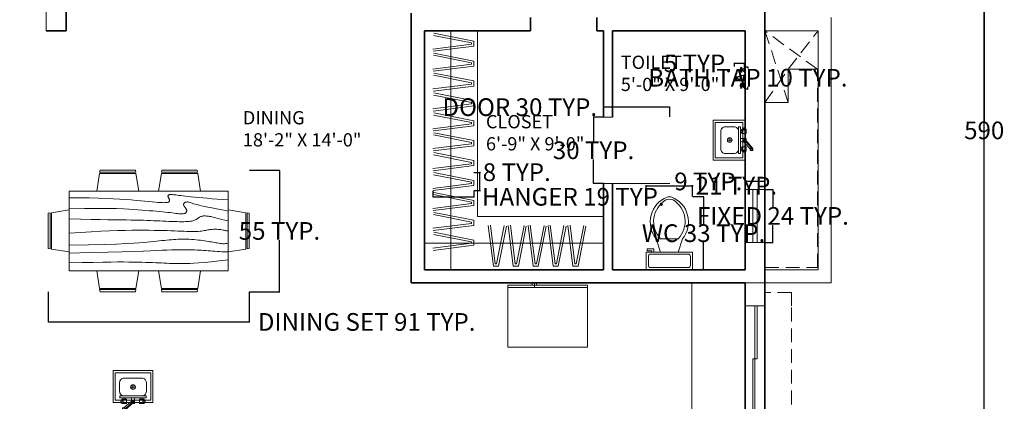
# Model space of a CAD drawing. Units: inches. Extents: x 3343 to 4790, y 1140 to 2641.
# Tile 9 of 10: x 4337 to 4782, y 2024 to 2196. Entities that reach past the tile are written whole.
import ezdxf

# ---------------------------------------------------------------- set-up
doc = ezdxf.new("R2010")
doc.units = ezdxf.units.IN
doc.header["$LTSCALE"] = 5
doc.header["$MEASUREMENT"] = 0
doc.linetypes.add('HIDDEN', pattern=[0.375, 0.25, -0.125])
for name, color, linetype, lineweight in [('A-ANNO-DIMS', 2, 'Continuous', 18), ('A-AREA-IDEN', 7, 'Continuous', 18), ('A-DOOR', 3, 'Continuous', 18), ('A-EQPM', 9, 'Continuous', 18), ('A-FLOR-CASE', 9, 'Continuous', 18), ('A-FLOR-FIXT', 9, 'Continuous', 18), ('A-FLOR-HIDN', 8, 'HIDDEN', 13), ('A-FLOR-SHFT', 8, 'Continuous', 18), ('A-FURN', 8, 'Continuous', 13), ('A-GLAZ', 4, 'Continuous', 18), ('A-WALL', 7, 'Continuous', 35)]:
    doc.layers.add(name, color=color, linetype=linetype, lineweight=lineweight)
doc.styles.get("Standard").update_dxf_attribs({"font": 'arial.ttf'})
doc.dimstyles.get("Standard").update_dxf_attribs({"dimtxt": 8, "dimasz": 0.18, "dimexe": 0.18, "dimexo": 0.0625, "dimgap": 0.09, "dimtad": 0, "dimtih": 1, "dimtoh": 1, "dimdec": 1, "dimzin": 0, "dimdsep": 46, "dimlunit": 3, "dimtxsty": 'Standard', "dimcen": 0.09, "dimadec": 0, "dimazin": 0, "dimtfac": 1, "dimtdec": 1, "dimtofl": 0, "dimtmove": 0, "dimatfit": 3, "dimfxl": 1, "dimtolj": 1, "dimtzin": 0, "dimarcsym": 0})

# ---------------------------------------------------------------- blocks, each defined once
blk = doc.blocks.new('Dining Set - 36 x 72 in.')
for p, q in [((-22, 27.5), (-22.1562, 26.50042)), ((-22, 27.5), (-6, 27.5)), ((-5.8437, 26.49966), (-6, 27.5)), ((6, 27.5), (5.8438, 26.50042)), ((6, 27.5), (22, 27.5)), ((22.1563, 26.49966), (22, 27.5)), ((-22.2343, 26.00059), (-23.4847, 17.99762)), ((-22.2304, 26), (-5.7608, 26)), ((-5.8416, 26.5), (-22.1534, 26.5)), ((-4.5152, 17.99762), (-5.7655, 25.99926)), ((5.7657, 26.00059), (4.5153, 17.99762)), ((5.7696, 26), (22.2392, 26)), ((22.1584, 26.5), (5.8466, 26.5)), ((23.4848, 17.99762), (22.2345, 25.99926)), ((36, 18), (-36, 18)), ((-36, 18), (-36, -18)), ((36, -18), (36, 18)), ((-44.0006, 8.23428), (-35.9976, 9.48474)), ((44.0006, 8.23428), (35.9976, 9.48474)), ((-45.5, 8), (-44.5004, 8.15617)), ((-45.5, 8), (-45.5, -8)), ((-44.5, -8.15843), (-44.5, 8.15338)), ((-44, 8.23041), (-44, -8.23915)), ((44, 8.23041), (44, -8.23915)), ((44.5, -8.15843), (44.5, 8.15338)), ((45.5, 8), (44.5005, 8.15617)), ((45.5, 8), (45.5, -8)), ((-44.4997, -8.15631), (-45.5, -8)), ((-35.9976, -9.48476), (-43.9993, -8.2345)), ((35.9976, -9.48476), (43.9993, -8.2345)), ((44.4997, -8.15631), (45.5, -8)), ((-36, -18), (36, -18)), ((-22.2343, -26.0006), (-23.4847, -17.99762)), ((-4.5152, -17.99762), (-5.7655, -25.99928)), ((5.7657, -26.0006), (4.5153, -17.99762)), ((23.4848, -17.99762), (22.2345, -25.99928)), ((-22.2304, -26), (-5.7608, -26)), ((-22, -27.5), (-22.1562, -26.50044)), ((-5.8416, -26.5), (-22.1534, -26.5)), ((-5.8437, -26.49967), (-6, -27.5)), ((5.7696, -26), (22.2392, -26)), ((6, -27.5), (5.8438, -26.50044)), ((22.1584, -26.5), (5.8466, -26.5)), ((22.1563, -26.49967), (22, -27.5)), ((-22, -27.5), (-6, -27.5)), ((6, -27.5), (22, -27.5))]:
    blk.add_line(p, q)
for points in [[(-36, 15), (-31.1772, 14.97754), (-26.8079, 14.91406), (-22.8538, 14.81543), (-19.276, 14.6875), (-16.0362, 14.53613), (-13.0957, 14.36718), (-10.4159, 14.18652), (-7.9583, 14), (-5.6904, 13.81315), (-3.6035, 13.63021), (-1.6954, 13.45508), (0.0365, 13.29166), (1.5945, 13.14388), (2.9811, 13.01562), (4.1988, 12.9108), (5.25, 12.83333), (6.1393, 12.78613), (6.8802, 12.76823), (7.4883, 12.77767), (7.9792, 12.8125), (8.3685, 12.87077), (8.6719, 12.95052), (8.9049, 13.0498), (9.0833, 13.16666), (9.2205, 13.29899), (9.3216, 13.44401), (9.3895, 13.59879), (9.4271, 13.76041), (9.4373, 13.92594), (9.4232, 14.09245), (9.3875, 14.257), (9.3333, 14.41666), (9.2638, 14.56917), (9.1836, 14.71484), (9.0975, 14.85465), (9.0104, 14.98958), (8.9272, 15.1206), (8.8529, 15.2487), (8.7922, 15.37483), (8.75, 15.5), (8.7305, 15.62467), (8.7344, 15.74739), (8.7617, 15.86621), (8.8125, 15.97916), (8.8867, 16.08431), (8.9844, 16.17968), (9.1055, 16.26334), (9.25, 16.33333), (9.4189, 16.38802), (9.6172, 16.42708), (9.8506, 16.45052), (10.125, 16.45833), (10.4463, 16.45052), (10.8203, 16.42708), (11.2529, 16.38802), (11.75, 16.33333), (12.3184, 16.26318), (12.9694, 16.17838), (13.7151, 16.07991), (14.5677, 15.96875), (15.5395, 15.84586), (16.6426, 15.71224), (17.8893, 15.56884), (19.2917, 15.41666), (20.859, 15.25667), (22.5879, 15.08984), (24.4721, 14.91715), (26.5052, 14.73958), (28.6809, 14.5581), (30.9929, 14.3737), (33.4347, 14.18733), (36, 14)], [(-36, 10), (-28.9766, 10.14274), (-23.1725, 10.20442), (-18.4241, 10.19775), (-14.5677, 10.13541), (-11.4399, 10.03011), (-8.877, 9.89453), (-6.7154, 9.74137), (-4.7917, 9.58333), (-2.9698, 9.43082), (-1.2246, 9.28515), (0.4415, 9.14534), (2.026, 9.01041), (3.5266, 8.87939), (4.9408, 8.7513), (6.266, 8.62516), (7.5, 8.5), (8.6411, 8.37549), (9.6914, 8.2539), (10.6538, 8.13818), (11.5312, 8.03125), (12.3267, 7.93603), (13.043, 7.85547), (13.6831, 7.79248), (14.25, 7.75), (14.7471, 7.7303), (15.1797, 7.73307), (15.5537, 7.75732), (15.875, 7.80208), (16.1494, 7.86637), (16.3828, 7.94922), (16.5811, 8.04964), (16.75, 8.16666), (16.8944, 8.29915), (17.0143, 8.44531), (17.1089, 8.60319), (17.1771, 8.77083), (17.218, 8.94629), (17.2305, 9.1276), (17.2137, 9.31282), (17.1667, 9.5), (17.0895, 9.6875), (16.987, 9.875), (16.8649, 10.0625), (16.7292, 10.25), (16.5856, 10.4375), (16.4401, 10.625), (16.2985, 10.8125), (16.1667, 11), (16.05, 11.18733), (15.9518, 11.3737), (15.8752, 11.5581), (15.8229, 11.73958), (15.798, 11.91715), (15.8034, 12.08984), (15.842, 12.25667), (15.9167, 12.41666), (16.0295, 12.56836), (16.1784, 12.70833), (16.3605, 12.83268), (16.5729, 12.9375), (16.8127, 13.01888), (17.0768, 13.07291), (17.3625, 13.0957), (17.6667, 13.08333), (17.9894, 13.03312), (18.3418, 12.94726), (18.7382, 12.82918), (19.1927, 12.68229), (19.7195, 12.51001), (20.3327, 12.31575), (21.0465, 12.10294), (21.875, 11.875), (22.8357, 11.63354), (23.959, 11.37304), (25.2786, 11.08618), (26.8282, 10.76562), (28.6414, 10.40405), (30.752, 9.99414), (33.1936, 9.52856), (36, 9)], [(-36, 5.5), (-30.7157, 5.3348), (-26.069, 5.20963), (-21.9946, 5.11767), (-18.4271, 5.05208), (-15.3009, 5.00602), (-12.5508, 4.97265), (-10.1112, 4.94515), (-7.9167, 4.91666), (-5.909, 4.88167), (-4.0586, 4.83984), (-2.3429, 4.79215), (-0.7396, 4.73958), (0.7739, 4.6831), (2.22, 4.6237), (3.6213, 4.56233), (5, 4.5), (6.373, 4.43782), (7.7344, 4.3776), (9.0723, 4.32129), (10.375, 4.27083), (11.6309, 4.22819), (12.8281, 4.19531), (13.9551, 4.17415), (15, 4.16666), (15.954, 4.17448), (16.819, 4.19791), (17.6001, 4.23698), (18.3021, 4.29166), (18.9299, 4.36198), (19.4883, 4.44791), (19.9823, 4.54948), (20.4167, 4.66666), (20.7969, 4.79899), (21.1302, 4.94401), (21.4245, 5.09879), (21.6875, 5.26041), (21.9271, 5.42594), (22.1511, 5.59245), (22.3672, 5.757), (22.5834, 5.91666), (22.8065, 6.06868), (23.0404, 6.21093), (23.2879, 6.34147), (23.5521, 6.45833), (23.8358, 6.55957), (24.142, 6.64323), (24.4735, 6.70735), (24.8334, 6.75), (25.2235, 6.76969), (25.642, 6.76692), (26.0858, 6.74267), (26.5521, 6.69791), (27.0379, 6.63362), (27.5404, 6.55078), (28.0565, 6.45036), (28.5834, 6.33333), (29.1242, 6.19987), (29.7071, 6.04687), (30.3661, 5.87044), (31.1354, 5.66666), (32.0493, 5.43164), (33.142, 5.16146), (34.4475, 4.85221), (36, 4.5)], [(-36, -1), (-30.7915, -0.6591), (-26.0195, -0.38216), (-21.6519, -0.16284), (-17.6563, 0.00521), (-14.0005, 0.12833), (-10.6523, 0.21289), (-7.5796, 0.26522), (-4.75, 0.29166), (-2.134, 0.29793), (0.2878, 0.28711), (2.5317, 0.26163), (4.6146, 0.22396), (6.5529, 0.17651), (8.3633, 0.12174), (10.0623, 0.06209), (11.6667, 0), (13.1899, -0.06201), (14.6341, -0.1211), (15.9982, -0.17432), (17.2813, -0.21875), (18.4823, -0.25147), (19.6003, -0.26953), (20.6343, -0.27002), (21.5834, -0.25), (22.4481, -0.20768), (23.2357, -0.14584), (23.9549, -0.06836), (24.6146, 0.02083), (25.2235, 0.11784), (25.7904, 0.21875), (26.3241, 0.31966), (26.8334, 0.41666), (27.3265, 0.50618), (27.8099, 0.58593), (28.2894, 0.65397), (28.7709, 0.70833), (29.2601, 0.74707), (29.763, 0.76823), (30.2855, 0.76985), (30.8334, 0.75), (31.4088, 0.70784), (31.9994, 0.64713), (32.589, 0.57275), (33.1615, 0.48958), (33.7008, 0.4025), (34.1908, 0.3164), (34.6153, 0.23616), (34.9584, 0.16666), (35.2099, 0.11165), (35.3848, 0.07031), (35.504, 0.04069), (35.5886, 0.02083), (35.6594, 0.00879), (35.7377, 0.0026), (35.8442, 0.00032), (36, 0)], [(-36, -6.5), (-27.1843, -6.31267), (-20.084, -6.1263), (-14.469, -5.9419), (-10.1094, -5.76042), (-6.7752, -5.58285), (-4.2363, -5.41016), (-2.2629, -5.24333), (-0.625, -5.08334), (0.8708, -4.93099), (2.2715, -4.78646), (3.5872, -4.64974), (4.8281, -4.52084), (6.0046, -4.39974), (7.127, -4.28646), (8.2053, -4.18099), (9.25, -4.08334), (10.2705, -3.99382), (11.2734, -3.91407), (12.2647, -3.84603), (13.25, -3.79167), (14.2354, -3.75293), (15.2266, -3.73177), (16.2295, -3.73015), (17.25, -3.75), (18.2912, -3.79248), (19.3451, -3.85547), (20.4009, -3.93604), (21.4479, -4.03125), (22.4754, -4.13819), (23.4727, -4.25391), (24.4289, -4.37549), (25.3334, -4.5), (26.1785, -4.62492), (26.9694, -4.74935), (27.7145, -4.87281), (28.4219, -4.99479), (29.1, -5.11483), (29.7572, -5.23242), (30.4016, -5.34709), (31.0417, -5.45834), (31.6837, -5.56437), (32.3262, -5.65821), (32.9658, -5.73153), (33.599, -5.77604), (34.2224, -5.78345), (34.8327, -5.74545), (35.4264, -5.65373), (36, -5.5)], [(-36, -10), (-26.4022, -9.81299), (-18.4675, -9.62891), (-11.9839, -9.45069), (-6.7396, -9.28125), (-2.5226, -9.12354), (0.8789, -8.98047), (3.6769, -8.85498), (6.0833, -8.75), (8.2767, -8.66765), (10.3021, -8.60677), (12.1712, -8.56543), (13.8958, -8.54167), (15.4876, -8.53353), (16.9583, -8.53907), (18.3197, -8.55632), (19.5834, -8.58334), (20.7616, -8.61841), (21.8685, -8.66081), (22.9188, -8.71004), (23.9271, -8.76563), (24.9081, -8.82707), (25.8763, -8.89388), (26.8465, -8.96558), (27.8334, -9.04167), (28.8474, -9.12118), (29.8828, -9.20117), (30.93, -9.27824), (31.9792, -9.34896), (33.0205, -9.40991), (34.0443, -9.45768), (35.0407, -9.48885), (36, -9.5)], [(-36, -14.5), (-30.0881, -14.33513), (-25.0332, -14.21224), (-20.7312, -14.12647), (-17.0781, -14.07292), (-13.97, -14.04671), (-11.3027, -14.04297), (-8.9724, -14.05681), (-6.875, -14.08334), (-4.9224, -14.11833), (-3.0905, -14.16016), (-1.3709, -14.20785), (0.2448, -14.26042), (1.7647, -14.3169), (3.1973, -14.3763), (4.5507, -14.43767), (5.8333, -14.5), (7.0554, -14.5621), (8.235, -14.62175), (9.3922, -14.67652), (10.5469, -14.72396), (11.7192, -14.76164), (12.929, -14.78711), (14.1965, -14.79794), (15.5417, -14.79167), (16.9933, -14.76424), (18.6152, -14.70508), (20.4804, -14.60197), (22.6615, -14.44271), (25.2312, -14.21509), (28.2624, -13.9069), (31.8277, -13.50594), (36, -13)]]:
    blk.add_lwpolyline(points)
blk = doc.blocks.new('Toilet - top')
for p, q in [((9.5, -6), (9.5, -2)), ((-10, -8.5), (-8, -8.5)), ((-10, -9.5), (-10, -8.5)), ((-8, -8.5), (-8, -8)), ((-7, -8), (-7, -9.5)), ((-4, -8), (-6, -14)), ((4, -8), (6, -14)), ((-7, -9.5), (-10, -9.5)), ((4, -14), (-4, -14))]:
    blk.add_line(p, q)
blk.add_lwpolyline([(10.5, -8), (10.5, 0), (-10.5, 0), (-10.5, -8)], close=True)
for points in [[(-9.5, -2), (-9.5, -6)], [(8.5, -1), (-8.5, -1)], [(-8.5, -7), (8.5, -7)]]:
    blk.add_lwpolyline(points)
for centre, radius, start, end in [((-8.62, -1.88), 0.884, 81.8699, 188.1301), ((8.62, -1.88), 0.884, 351.8699, 98.1301), ((-8.62, -6.12), 0.884, 171.8699, 278.1301), ((8.62, -6.12), 0.884, 261.8699, 8.1301), ((3.52, -21.58), 12.17, 141.4691, 247.9714), ((4.2, -21.82), 11.33, 136.3677, 238.9468), ((-3.52, -21.58), 12.17, 292.0284, 38.5307), ((-4.2, -21.82), 11.33, 301.053, 43.6321), ((0, -27.88), 4, 245.7318, 294.2682), ((0, -29), 4, 254.8605, 285.1395)]:
    blk.add_arc(centre, radius, start, end)
blk = doc.blocks.new('Faucet - Bathroom front')
for p, q in [((-5, 0), (-2.25, 0)), ((-4.5087, 0.25), (-2.7408, 0.25)), ((-4, 1.625), (-4.25, 1.625)), ((-4, 1.375), (-4.25, 1.375)), ((-3.1442, 0.75), (-4.0979, 0.75)), ((-3.25, 1.625), (-3, 1.625)), ((-3.25, 1.375), (-3, 1.375)), ((-1.5, 0), (1.5, 0)), ((-1, 0.5), (1, 0.5)), ((-0.5, 4.25), (0.5, 4.25)), ((0.5, 3.75), (-0.5, 3.75)), ((-0.5, 3), (0.5, 3)), ((0.5, 2), (-0.5, 2)), ((-0.25, 3), (-0.25, 3.5)), ((0.25, 3.5), (0.25, 3)), ((2.25, 0), (5, 0)), ((2.7413, 0.25), (4.5092, 0.25)), ((3.25, 1.625), (3, 1.625)), ((3.25, 1.375), (3, 1.375)), ((4.1058, 0.75), (3.1521, 0.75)), ((4, 1.625), (4.25, 1.625)), ((4, 1.375), (4.25, 1.375))]:
    blk.add_line(p, q)
for points in [[(-0.25, 4.5), (0.25, 4.5)], [(-0.5, 3.75), (-0.5, 4.25)], [(0.25, 3.5), (-0.25, 3.5)], [(0.5, 4.25), (0.5, 3.75)]]:
    blk.add_lwpolyline(points)
for points in [[(-4, 1), (-4, 2), (-3.25, 2), (-3.25, 1)], [(3.25, 1), (3.25, 2), (4, 2), (4, 1)]]:
    blk.add_lwpolyline(points, close=True)
for centre in [(-4.5, 1.5), (-3.625, 1.5), (-2.75, 1.5), (2.75, 1.5), (3.625, 1.5), (4.5, 1.5)]:
    blk.add_circle(centre, 0.2795)
for centre, radius, start, end in [((-0.2575, 4.2575), 0.2426, 88.22243, 181.7776), ((0.2575, 4.2575), 0.2426, 358.2224, 91.77757), ((-5.375, 1.375), 1.4252, 285.2551, 344.7449), ((-1.875, 1.375), 1.4252, 195.2551, 254.7449), ((-0.7962, -0.2038), 0.7327, 106.1502, 163.8498), ((3, 1), 4.0311, 150.2551, 187.125), ((0.6413, 2.5), 1.246, 156.3417, 203.6583), ((-0.2575, 3.7425), 0.2426, 178.2224, 271.7776), ((0.2575, 3.7425), 0.2426, 268.2224, 1.777565), ((-3, 1), 4.0311, 352.875, 29.74488), ((-0.6413, 2.5), 1.246, 336.3417, 23.65835), ((0.7962, -0.2038), 0.7327, 16.1502, 73.84979), ((1.875, 1.375), 1.4252, 285.2551, 344.7449), ((5.375, 1.375), 1.4252, 195.2551, 254.7449)]:
    blk.add_arc(centre, radius, start, end)
blk = doc.blocks.new('Faucet - kit sink front')
for p, q in [((-0.25, 3), (3.75, 6.5)), ((3.75, 6), (-0.25, 2.5)), ((4.1921, 5.5041), (0.75, 2.5)), ((3.75, 6), (3.75, 6.5)), ((3.75, 6.5), (4.75, 6.5)), ((3.75, 5.5), (3.75, 6)), ((4.75, 6), (3.75, 6)), ((4.75, 5.5), (3.75, 5.5)), ((4.75, 6.5), (4.75, 6)), ((4.75, 6), (4.75, 5.5)), ((-4.5, 1), (-4.5, 1.5)), ((-3.5, 1.5), (-3.5, 1)), ((-0.75, 3.5), (0.3192, 3.5)), ((-0.75, 1), (-0.75, 3.5)), ((-0.25, 2.5), (-0.25, 3)), ((0.75, 2.5), (-0.25, 2.5)), ((0.75, 2.5), (0.75, 1)), ((3.5, 1.5), (3.5, 1)), ((4.5, 1), (4.5, 1.5))]:
    blk.add_line(p, q)
for points in [[(-6, 0), (-6, 1), (6, 1), (6, 0)], [(-5.5, 2.5), (-5.5, 3.25), (-4.5, 3.25), (-4.5, 2.5)], [(5.5, 2.5), (5.5, 3.25), (4.5, 3.25), (4.5, 2.5)]]:
    blk.add_lwpolyline(points, close=True)
for points in [[(-5, 3.2513), (-5, 3.5), (-3, 3.5), (-3, 1.5), (-5, 1.5), (-5, 2.5)], [(5, 3.2513), (5, 3.5), (3, 3.5), (3, 1.5), (5, 1.5), (5, 2.5)]]:
    blk.add_lwpolyline(points)
blk = doc.blocks.new('Refrigerator-2 door - 36 in top')
for p, q in [((0, -26.999999), (36, -26.999999)), ((11, -27.999999), (11, -28.999999)), ((11, -28.999999), (13, -28.999999)), ((12, -26.999999), (12, -28.999999)), ((13, -28.999999), (13, -27.999999))]:
    blk.add_line(p, q)
blk.add_lwpolyline([(0, -27.999999), (0, 0), (36, 0), (36, -27.999999)], close=True)
blk = doc.blocks.new('SINK-BOWL-WITH-DRAIN')
for p, q in [((8.58, 9.03), (6.47, 9.03)), ((7.52, 10.09), (7.52, 7.97))]:
    blk.add_line(p, q)
for points in [[(14.44, 0), (0, 0), (0, 18.06), (14.44, 18.06)], [(1, 1), (1, 17.06), (13.44, 17.06), (13.44, 1)]]:
    blk.add_lwpolyline(points, close=True)
blk.add_lwpolyline([(9.44, 15.06), (5.44, 15.06, 0.414214), (3.44, 13.06), (3.44, 5, 0.414214), (5.44, 3), (9.44, 3, 0.414214), (11.44, 5), (11.44, 13.06, 0.414214)], format="xyb", close=True)
blk.add_circle((7.52, 9.03), 1.06)
blk = doc.blocks.new('WINDOW-48IN-SLIDING-JAMB9')
for p, q in [((0, 9), (0, 0)), ((48, 9), (48, 0)), ((0, 5.5), (24, 5.5)), ((0, 4.5), (48, 4.5)), ((24, 5.5), (24, 3.5)), ((24, 3.5), (48, 3.5))]:
    blk.add_line(p, q)
blk = doc.blocks.new('WINDOW-24IN-FIXED')
for p, q in [((0, 9), (0, 0)), ((24, 9), (24, 0)), ((0, 5.5), (24, 5.5)), ((0, 3.5), (24, 3.5))]:
    blk.add_line(p, q)
blk = doc.blocks.new('DOOR-36IN-6IN-JAMB')
for p, q in [((0, 30), (0, 36)), ((36, 30), (36, 36)), ((36, 36), (36, 0))]:
    blk.add_line(p, q)
blk = doc.blocks.new('DOOR-30IN-4IN-JAMB')
for p, q in [((30, 30), (0, 30)), ((26, 30), (30, 30)), ((26, 0), (30, 0))]:
    blk.add_line(p, q)
blk = doc.blocks.new('WARDROBE-HANGER')
for points in [[(0.22, 7.19), (17.51, 3.78), (17.51, 3.18), (0, 0.99)], [(0.41, 8.17), (18.51, 4.61), (18.51, 2.3), (0.12, 0)]]:
    blk.add_lwpolyline(points)
blk = doc.blocks.new('*D29')
at = {"layer": 'A-ANNO-DIMS', "color": 0, "lineweight": -2, "ltscale": 5, "transparency": 16777216}
for p, q in [((4523.96, 2118.86), (4523.96, 2115.96)), ((4524.14, 2116.14), (4542.3, 2116.14)), ((4542.48, 2118.86), (4542.48, 2115.96)), ((4542.48, 2116.14), (4542.66, 2116.14))]:
    blk.add_line(p, q, dxfattribs=at)
at = {"layer": 'A-ANNO-DIMS', "color": 0, "ltscale": 5, "transparency": 16777216}
for points in [[(4524.14, 2116.17), (4524.14, 2116.11), (4523.96, 2116.14)], [(4542.3, 2116.17), (4542.3, 2116.11), (4542.48, 2116.14)]]:
    blk.add_solid(points, dxfattribs=at)
at = {"layer": 'Defpoints', "color": 0, "ltscale": 5, "transparency": 16777216}
for p in [(4523.96, 2118.92), (4542.48, 2118.92), (4542.48, 2116.14)]:
    blk.add_point(p, dxfattribs=at)
at = {"layer": 'A-ANNO-DIMS', "color": 0, "ltscale": 5, "transparency": 16777216, "insert": (4587.46, 2116.14), "char_height": 8, "attachment_point": 5}
blk.add_mtext('\\A1;HANGER 19 TYP.', dxfattribs=at)
blk = doc.blocks.new('*D30')
at = {"layer": 'A-ANNO-DIMS', "color": 0, "lineweight": -2, "ltscale": 5, "transparency": 16777216}
for p, q in [((4542.54, 2127.09), (4545.43, 2127.09)), ((4545.25, 2127.09), (4545.25, 2127.27)), ((4545.25, 2127.27), (4545.43, 2127.27)), ((4545.25, 2119.1), (4545.25, 2126.91)), ((4542.54, 2118.92), (4545.43, 2118.92))]:
    blk.add_line(p, q, dxfattribs=at)
at = {"layer": 'A-ANNO-DIMS', "color": 0, "ltscale": 5, "transparency": 16777216}
for points in [[(4545.22, 2126.91), (4545.28, 2126.91), (4545.25, 2127.09)], [(4545.22, 2119.1), (4545.28, 2119.1), (4545.25, 2118.92)]]:
    blk.add_solid(points, dxfattribs=at)
at = {"layer": 'Defpoints', "color": 0, "ltscale": 5, "transparency": 16777216}
for p in [(4542.48, 2127.09), (4545.25, 2127.09), (4542.48, 2118.92)]:
    blk.add_point(p, dxfattribs=at)
at = {"layer": 'A-ANNO-DIMS', "color": 0, "ltscale": 5, "transparency": 16777216, "insert": (4561.89, 2127.27), "char_height": 8, "attachment_point": 5}
blk.add_mtext('\\A1;8 TYP.', dxfattribs=at)
blk = doc.blocks.new('*D39')
at = {"layer": 'A-ANNO-DIMS', "color": 0, "lineweight": -2, "ltscale": 5, "transparency": 16777216}
for p, q in [((4664.99, 2174.96), (4666.61, 2174.96)), ((4666.43, 2174.78), (4666.43, 2174.13)), ((4664.99, 2164.96), (4666.61, 2164.96)), ((4666.43, 2165.14), (4666.43, 2165.78))]:
    blk.add_line(p, q, dxfattribs=at)
at = {"layer": 'A-ANNO-DIMS', "color": 0, "ltscale": 5, "transparency": 16777216}
for points in [[(4666.4, 2174.78), (4666.46, 2174.78), (4666.43, 2174.96)], [(4666.4, 2165.14), (4666.46, 2165.14), (4666.43, 2164.96)]]:
    blk.add_solid(points, dxfattribs=at)
at = {"layer": 'Defpoints', "color": 0, "ltscale": 5, "transparency": 16777216}
for p in [(4664.93, 2174.96), (4666.43, 2174.96), (4664.93, 2164.96)]:
    blk.add_point(p, dxfattribs=at)
at = {"layer": 'A-ANNO-DIMS', "color": 0, "ltscale": 5, "transparency": 16777216, "insert": (4666.43, 2169.96), "char_height": 8, "attachment_point": 5}
blk.add_mtext('\\A1;BATH TAP 10 TYP.', dxfattribs=at)
blk = doc.blocks.new('*D40')
at = {"layer": 'A-ANNO-DIMS', "color": 0, "lineweight": -2, "ltscale": 5, "transparency": 16777216}
for p, q in [((4660.42, 2176.46), (4660.24, 2176.46)), ((4660.42, 2175.02), (4660.42, 2176.64)), ((4664.75, 2176.46), (4660.6, 2176.46)), ((4664.93, 2175.02), (4664.93, 2176.64))]:
    blk.add_line(p, q, dxfattribs=at)
at = {"layer": 'A-ANNO-DIMS', "color": 0, "ltscale": 5, "transparency": 16777216}
for points in [[(4660.6, 2176.49), (4660.6, 2176.43), (4660.42, 2176.46)], [(4664.75, 2176.49), (4664.75, 2176.43), (4664.93, 2176.46)]]:
    blk.add_solid(points, dxfattribs=at)
at = {"layer": 'Defpoints', "color": 0, "ltscale": 5, "transparency": 16777216}
for p in [(4660.42, 2176.46), (4660.42, 2174.96), (4664.93, 2174.96)]:
    blk.add_point(p, dxfattribs=at)
at = {"layer": 'A-ANNO-DIMS', "color": 0, "ltscale": 5, "transparency": 16777216, "insert": (4643.79, 2176.46), "char_height": 8, "attachment_point": 5}
blk.add_mtext('\\A1;5 TYP.', dxfattribs=at)
blk = doc.blocks.new('*D41')
at = {"layer": 'A-ANNO-DIMS', "color": 0, "lineweight": -2, "ltscale": 5, "transparency": 16777216}
for p, q in [((4641.48, 2116.21), (4646.55, 2116.21)), ((4646.37, 2116.03), (4646.37, 2103.91)), ((4646.37, 2083.34), (4646.37, 2095.45)), ((4641.48, 2083.16), (4646.55, 2083.16))]:
    blk.add_line(p, q, dxfattribs=at)
at = {"layer": 'A-ANNO-DIMS', "color": 0, "ltscale": 5, "transparency": 16777216}
for points in [[(4646.34, 2116.03), (4646.4, 2116.03), (4646.37, 2116.21)], [(4646.34, 2083.34), (4646.4, 2083.34), (4646.37, 2083.16)]]:
    blk.add_solid(points, dxfattribs=at)
at = {"layer": 'Defpoints', "color": 0, "ltscale": 5, "transparency": 16777216}
for p in [(4641.42, 2116.21), (4641.42, 2083.16), (4646.37, 2083.16)]:
    blk.add_point(p, dxfattribs=at)
at = {"layer": 'A-ANNO-DIMS', "color": 0, "ltscale": 5, "transparency": 16777216, "insert": (4646.37, 2099.68), "char_height": 8, "attachment_point": 5}
blk.add_mtext('\\A1;WC 33 TYP.', dxfattribs=at)
blk = doc.blocks.new('*D42')
at = {"layer": 'A-ANNO-DIMS', "color": 0, "lineweight": -2, "ltscale": 5, "transparency": 16777216}
for p, q in [((4620.42, 2116.27), (4620.42, 2121.34)), ((4620.6, 2121.16), (4641.24, 2121.16)), ((4641.42, 2116.27), (4641.42, 2121.34)), ((4641.42, 2121.16), (4641.6, 2121.16))]:
    blk.add_line(p, q, dxfattribs=at)
at = {"layer": 'A-ANNO-DIMS', "color": 0, "ltscale": 5, "transparency": 16777216}
for points in [[(4620.6, 2121.19), (4620.6, 2121.13), (4620.42, 2121.16)], [(4641.24, 2121.19), (4641.24, 2121.13), (4641.42, 2121.16)]]:
    blk.add_solid(points, dxfattribs=at)
at = {"layer": 'Defpoints', "color": 0, "ltscale": 5, "transparency": 16777216}
for p in [(4641.42, 2121.16), (4620.42, 2116.21), (4641.42, 2116.21)]:
    blk.add_point(p, dxfattribs=at)
at = {"layer": 'A-ANNO-DIMS', "color": 0, "ltscale": 5, "transparency": 16777216, "insert": (4661.23, 2121.16), "char_height": 8, "attachment_point": 5}
blk.add_mtext('\\A1;21 TYP.', dxfattribs=at)
blk = doc.blocks.new('*D49')
at = {"layer": 'A-ANNO-DIMS', "color": 0, "lineweight": -2, "ltscale": 5, "transparency": 16777216}
for p, q in [((4674.19, 2119.48), (4677.91, 2119.48)), ((4677.73, 2119.3), (4677.73, 2111.59)), ((4677.73, 2095.66), (4677.73, 2103.37)), ((4674.19, 2095.48), (4677.91, 2095.48))]:
    blk.add_line(p, q, dxfattribs=at)
at = {"layer": 'A-ANNO-DIMS', "color": 0, "ltscale": 5, "transparency": 16777216}
for points in [[(4677.7, 2119.3), (4677.76, 2119.3), (4677.73, 2119.48)], [(4677.7, 2095.66), (4677.76, 2095.66), (4677.73, 2095.48)]]:
    blk.add_solid(points, dxfattribs=at)
at = {"layer": 'Defpoints', "color": 0, "ltscale": 5, "transparency": 16777216}
for p in [(4674.13, 2119.48), (4677.73, 2119.48), (4674.13, 2095.48)]:
    blk.add_point(p, dxfattribs=at)
at = {"layer": 'A-ANNO-DIMS', "color": 0, "ltscale": 5, "transparency": 16777216, "insert": (4677.73, 2107.48), "char_height": 8, "attachment_point": 5}
blk.add_mtext('\\A1;FIXED 24 TYP.', dxfattribs=at)
blk = doc.blocks.new('*D50')
at = {"layer": 'A-ANNO-DIMS', "color": 0, "lineweight": -2, "ltscale": 5, "transparency": 16777216}
for p, q in [((4665.13, 2123.08), (4664.95, 2123.08)), ((4665.13, 2119.54), (4665.13, 2123.26)), ((4673.95, 2123.08), (4665.31, 2123.08)), ((4674.13, 2119.54), (4674.13, 2123.26))]:
    blk.add_line(p, q, dxfattribs=at)
at = {"layer": 'A-ANNO-DIMS', "color": 0, "ltscale": 5, "transparency": 16777216}
for points in [[(4665.31, 2123.11), (4665.31, 2123.05), (4665.13, 2123.08)], [(4673.95, 2123.11), (4673.95, 2123.05), (4674.13, 2123.08)]]:
    blk.add_solid(points, dxfattribs=at)
at = {"layer": 'Defpoints', "color": 0, "ltscale": 5, "transparency": 16777216}
for p in [(4665.13, 2123.08), (4665.13, 2119.48), (4674.13, 2119.48)]:
    blk.add_point(p, dxfattribs=at)
at = {"layer": 'A-ANNO-DIMS', "color": 0, "ltscale": 5, "transparency": 16777216, "insert": (4648.5, 2123.08), "char_height": 8, "attachment_point": 5}
blk.add_mtext('\\A1;9 TYP.', dxfattribs=at)
blk = doc.blocks.new('*D53')
at = {"layer": 'A-ANNO-DIMS', "color": 0, "lineweight": -2, "ltscale": 5, "transparency": 16777216}
for p, q in [((4601.13, 2156.66), (4600.95, 2156.66)), ((4601.13, 2152.22), (4601.13, 2156.84)), ((4630.95, 2156.66), (4601.31, 2156.66)), ((4631.13, 2152.22), (4631.13, 2156.84))]:
    blk.add_line(p, q, dxfattribs=at)
at = {"layer": 'A-ANNO-DIMS', "color": 0, "ltscale": 5, "transparency": 16777216}
for points in [[(4601.31, 2156.69), (4601.31, 2156.63), (4601.13, 2156.66)], [(4630.95, 2156.69), (4630.95, 2156.63), (4631.13, 2156.66)]]:
    blk.add_solid(points, dxfattribs=at)
at = {"layer": 'Defpoints', "color": 0, "ltscale": 5, "transparency": 16777216}
for p in [(4601.13, 2156.66), (4601.13, 2152.16), (4631.13, 2152.16)]:
    blk.add_point(p, dxfattribs=at)
at = {"layer": 'A-ANNO-DIMS', "color": 0, "ltscale": 5, "transparency": 16777216, "insert": (4563.27, 2156.66), "char_height": 8, "attachment_point": 5}
blk.add_mtext('\\A1;DOOR 30 TYP.', dxfattribs=at)
blk = doc.blocks.new('*D54')
at = {"layer": 'A-ANNO-DIMS', "color": 0, "lineweight": -2, "ltscale": 5, "transparency": 16777216}
for p, q in [((4601.07, 2152.16), (4596.45, 2152.16)), ((4596.63, 2151.98), (4596.63, 2141.34)), ((4596.63, 2122.34), (4596.63, 2132.98)), ((4601.07, 2122.16), (4596.45, 2122.16))]:
    blk.add_line(p, q, dxfattribs=at)
at = {"layer": 'A-ANNO-DIMS', "color": 0, "ltscale": 5, "transparency": 16777216}
for points in [[(4596.6, 2151.98), (4596.66, 2151.98), (4596.63, 2152.16)], [(4596.6, 2122.34), (4596.66, 2122.34), (4596.63, 2122.16)]]:
    blk.add_solid(points, dxfattribs=at)
at = {"layer": 'Defpoints', "color": 0, "ltscale": 5, "transparency": 16777216}
for p in [(4601.13, 2152.16), (4596.63, 2122.16), (4601.13, 2122.16)]:
    blk.add_point(p, dxfattribs=at)
at = {"layer": 'A-ANNO-DIMS', "color": 0, "ltscale": 5, "transparency": 16777216, "insert": (4596.63, 2137.16), "char_height": 8, "attachment_point": 5}
blk.add_mtext('\\A1;30 TYP.', dxfattribs=at)
blk = doc.blocks.new('*D67')
at = {"layer": 'A-ANNO-DIMS', "color": 0, "lineweight": -2, "ltscale": 5, "transparency": 16777216}
for p, q in [((4349.95, 2073.14), (4349.95, 2059.37)), ((4440.95, 2073.14), (4440.95, 2059.37)), ((4350.13, 2059.55), (4440.77, 2059.55)), ((4440.95, 2059.55), (4441.13, 2059.55))]:
    blk.add_line(p, q, dxfattribs=at)
at = {"layer": 'A-ANNO-DIMS', "color": 0, "ltscale": 5, "transparency": 16777216}
for points in [[(4350.13, 2059.58), (4350.13, 2059.52), (4349.95, 2059.55)], [(4440.77, 2059.58), (4440.77, 2059.52), (4440.95, 2059.55)]]:
    blk.add_solid(points, dxfattribs=at)
at = {"layer": 'Defpoints', "color": 0, "ltscale": 5, "transparency": 16777216}
for p in [(4349.95, 2073.2), (4440.95, 2073.2), (4440.95, 2059.55)]:
    blk.add_point(p, dxfattribs=at)
at = {"layer": 'A-ANNO-DIMS', "color": 0, "ltscale": 5, "transparency": 16777216, "insert": (4494.02, 2059.55), "char_height": 8, "attachment_point": 5}
blk.add_mtext('\\A1;DINING SET 91 TYP.', dxfattribs=at)
blk = doc.blocks.new('*D68')
at = {"layer": 'A-ANNO-DIMS', "color": 0, "lineweight": -2, "ltscale": 5, "transparency": 16777216}
for p, q in [((4441.01, 2128.2), (4454.78, 2128.2)), ((4454.6, 2128.02), (4454.6, 2104.86)), ((4454.6, 2073.38), (4454.6, 2096.54)), ((4441.01, 2073.2), (4454.78, 2073.2))]:
    blk.add_line(p, q, dxfattribs=at)
at = {"layer": 'A-ANNO-DIMS', "color": 0, "ltscale": 5, "transparency": 16777216}
for points in [[(4454.57, 2128.02), (4454.63, 2128.02), (4454.6, 2128.2)], [(4454.57, 2073.38), (4454.63, 2073.38), (4454.6, 2073.2)]]:
    blk.add_solid(points, dxfattribs=at)
at = {"layer": 'Defpoints', "color": 0, "ltscale": 5, "transparency": 16777216}
for p in [(4440.95, 2128.2), (4454.6, 2128.2), (4440.95, 2073.2)]:
    blk.add_point(p, dxfattribs=at)
at = {"layer": 'A-ANNO-DIMS', "color": 0, "ltscale": 5, "transparency": 16777216, "insert": (4454.6, 2100.7), "char_height": 8, "attachment_point": 5}
blk.add_mtext('\\A1;55 TYP.', dxfattribs=at)
blk = doc.blocks.new('*D87')
at = {"layer": 'A-ANNO-DIMS', "color": 0, "lineweight": -2, "ltscale": 5, "transparency": 16777216}
for p, q in [((3977.19, 2566.16), (4773.46, 2566.16)), ((4773.28, 2565.98), (4773.28, 2294.34)), ((4773.28, 2014.34), (4773.28, 2285.99)), ((3977.19, 2014.16), (4773.46, 2014.16))]:
    blk.add_line(p, q, dxfattribs=at)
at = {"layer": 'A-ANNO-DIMS', "color": 0, "ltscale": 5, "transparency": 16777216}
for points in [[(4773.25, 2565.98), (4773.31, 2565.98), (4773.28, 2566.16)], [(4773.25, 2014.34), (4773.31, 2014.34), (4773.28, 2014.16)]]:
    blk.add_solid(points, dxfattribs=at)
at = {"layer": 'Defpoints', "color": 0, "ltscale": 5, "transparency": 16777216}
for p in [(3977.13, 2566.16), (3977.13, 2014.16), (4773.28, 2014.16)]:
    blk.add_point(p, dxfattribs=at)
at = {"layer": 'A-ANNO-DIMS', "color": 0, "ltscale": 5, "transparency": 16777216, "insert": (4773.28, 2290.16), "char_height": 8, "attachment_point": 5}
blk.add_mtext('\\A1;552', dxfattribs=at)
blk = doc.blocks.new('*D88')
at = {"layer": 'A-ANNO-DIMS', "color": 0, "lineweight": -2, "ltscale": 5, "transparency": 16777216}
for p, q in [((4674.19, 2441.16), (4773.46, 2441.16)), ((4773.28, 2440.98), (4773.28, 2150.34)), ((4773.28, 1851.34), (4773.28, 2141.99)), ((4674.19, 1851.16), (4773.46, 1851.16))]:
    blk.add_line(p, q, dxfattribs=at)
at = {"layer": 'A-ANNO-DIMS', "color": 0, "ltscale": 5, "transparency": 16777216}
for points in [[(4773.25, 2440.98), (4773.31, 2440.98), (4773.28, 2441.16)], [(4773.25, 1851.34), (4773.31, 1851.34), (4773.28, 1851.16)]]:
    blk.add_solid(points, dxfattribs=at)
at = {"layer": 'Defpoints', "color": 0, "ltscale": 5, "transparency": 16777216}
for p in [(4674.13, 2441.16), (4773.28, 2441.16), (4674.13, 1851.16)]:
    blk.add_point(p, dxfattribs=at)
at = {"layer": 'A-ANNO-DIMS', "color": 0, "ltscale": 5, "transparency": 16777216, "insert": (4773.28, 2146.16), "char_height": 8, "attachment_point": 5}
blk.add_mtext('\\A1;590', dxfattribs=at)

msp = doc.modelspace()

# ---------------------------------------------------------------- linework, layer by layer
at = {"layer": 'A-FLOR-CASE'}
for p, q in [((4544.13, 2191.161), (4532.13, 2191.161)), ((4532.13, 2191.161), (4532.13, 2083.161)), ((4544.13, 2191.161), (4544.13, 2107.161)), ((4544.13, 2107.161), (4601.13, 2107.161)), ((4601.13, 2095.161), (4520.13, 2095.161)), ((4601.13, 2083.161), (4601.13, 2095.161)), ((4641.13, 2077.161), (4641.13, 1948.161))]:
    msp.add_line(p, q, dxfattribs=at)
at = {"layer": 'A-FLOR-FIXT'}
for p, q in [((4388.365, 2029.013), (4388.365, 2031.133)), ((4389.424, 2030.073), (4387.305, 2030.073))]:
    msp.add_line(p, q, dxfattribs=at)
for points in [[(4379.334, 2023.161), (4379.334, 2037.598), (4397.396, 2037.598), (4397.396, 2023.161)], [(4380.334, 2036.598), (4396.396, 2036.598), (4396.396, 2024.161), (4380.334, 2024.161)]]:
    msp.add_lwpolyline(points, close=True, dxfattribs=at)
msp.add_lwpolyline([(4394.396, 2028.161), (4394.396, 2032.161, 0.4142136), (4392.396, 2034.161), (4384.334, 2034.161, 0.4142136), (4382.334, 2032.161), (4382.334, 2028.161, 0.4142136), (4384.334, 2026.161), (4392.396, 2026.161, 0.4142136)], format="xyb", close=True, dxfattribs=at)
msp.add_circle((4388.365, 2030.073), 1.06, dxfattribs=at)
at = {"layer": 'A-FLOR-HIDN', "ltscale": 5}
for p, q in [((4697.836, 2173.811), (4674.13, 2191.161)), ((4674.13, 2191.161), (4684.646, 2158.83)), ((4684.646, 2173.811), (4698.13, 2191.161)), ((4674.13, 2158.83), (4684.646, 2173.811)), ((4697.836, 2084.131), (4697.836, 2173.811)), ((4674.13, 2084.131), (4697.836, 2084.131)), ((4686.13, 2072.896), (4674.13, 2072.896)), ((4686.13, 2066.896), (4686.13, 2072.896)), ((4686.13, 2012.896), (4686.13, 2066.896))]:
    msp.add_line(p, q, dxfattribs=at)
at = {"layer": 'A-FLOR-SHFT'}
for p, q in [((4704.13, 2197.161), (4704.13, 2077.161)), ((4674.13, 2191.161), (4698.13, 2191.161)), ((4698.13, 2191.161), (4698.13, 2083.161)), ((4698.13, 2173.811), (4684.646, 2173.811)), ((4684.646, 2173.811), (4684.646, 2158.83)), ((4684.646, 2158.83), (4674.13, 2158.83)), ((4674.13, 2083.161), (4698.13, 2083.161)), ((4665.13, 2077.161), (4674.13, 2077.161)), ((4674.13, 2077.161), (4704.13, 2077.161))]:
    msp.add_line(p, q, dxfattribs=at)
at = {"layer": 'A-WALL'}
for p, q in [((4674.13, 2441.161), (4674.13, 1851.161)), ((4358.13, 2336.161), (4358.13, 2191.161)), ((4514.13, 2199.161), (4514.13, 2191.161)), ((4568.13, 2191.161), (4568.13, 2197.161)), ((4598.13, 2191.161), (4598.13, 2197.161)), ((4349.13, 2191.161), (4358.13, 2191.161)), ((4514.13, 2191.161), (4514.13, 2077.161)), ((4520.13, 2191.161), (4520.13, 2083.161)), ((4520.13, 2191.161), (4568.13, 2191.161)), ((4520.13, 2191.161), (4520.13, 2083.161)), ((4598.13, 2191.161), (4601.13, 2191.161)), ((4601.13, 2191.161), (4601.13, 2152.161)), ((4605.13, 2191.161), (4605.13, 2152.161)), ((4605.13, 2191.161), (4665.13, 2191.161)), ((4665.13, 2191.161), (4665.13, 2083.161)), ((4601.13, 2122.161), (4601.13, 2083.161)), ((4605.13, 2122.161), (4605.13, 2083.161)), ((4520.13, 2083.161), (4601.13, 2083.161)), ((4605.13, 2083.161), (4665.13, 2083.161)), ((4514.13, 2077.161), (4665.13, 2077.161)), ((4605.13, 2077.161), (4665.13, 2077.161)), ((4665.13, 2077.161), (4665.13, 1924.161))]:
    msp.add_line(p, q, dxfattribs=at)

# ---------------------------------------------------------------- block references
at = {"layer": 'A-DOOR', "extrusion": (0, 0, -1), "zscale": -1, "rotation": 180}
msp.add_blockref('DOOR-36IN-6IN-JAMB', (-4313.13, 2227.161), dxfattribs=at)
at = {"layer": 'A-DOOR', "rotation": 180}
msp.add_blockref('DOOR-30IN-4IN-JAMB', (4631.129, 2152.161), dxfattribs=at)
at = {"layer": 'A-EQPM', "xscale": -1, "rotation": 180}
msp.add_blockref('Refrigerator-2 door - 36 in top', (4557.887, 2048.161), dxfattribs=at)
at = {"layer": 'A-FLOR-CASE'}
for p in [(4523.963, 2181.918), (4523.963, 2172.918), (4523.963, 2163.918), (4523.963, 2154.918), (4523.963, 2145.918), (4523.963, 2136.918), (4523.963, 2127.918), (4523.963, 2118.918), (4523.963, 2109.918), (4523.963, 2100.918), (4523.963, 2091.918)]:
    msp.add_blockref('WARDROBE-HANGER', p, dxfattribs=at)
for p, rotation in [((4549.03, 2103.328), 270.0000000000094), ((4558.03, 2103.328), 270.0000000000045), ((4567.03, 2103.328), 269.9999999999996), ((4576.03, 2103.328), 269.9999999999996), ((4585.03, 2103.328), 270.0000000000045)]:
    msp.add_blockref('WARDROBE-HANGER', p, dxfattribs=dict(at, rotation=rotation))
at = {"layer": 'A-FLOR-FIXT'}
for name, p, rotation in [('Faucet - Bathroom front', (4664.926, 2169.958), 90), ('Faucet - kit sink front', (4662.13, 2141.74), 270), ('Faucet - kit sink front', (4388.365, 2026.161), 180)]:
    msp.add_blockref(name, p, dxfattribs=dict(at, rotation=rotation))
msp.add_blockref('SINK-BOWL-WITH-DRAIN', (4650.693, 2132.709), dxfattribs=at)
at = {"layer": 'A-FLOR-FIXT', "xscale": -1, "rotation": 180}
msp.add_blockref('Toilet - top', (4630.918, 2083.161), dxfattribs=at)
at = {"layer": 'A-FURN'}
msp.add_blockref('Dining Set - 36 x 72 in.', (4395.446, 2100.702), dxfattribs=at)
at = {"layer": 'A-GLAZ'}
for name, p, rotation in [('WINDOW-24IN-FIXED', (4674.13, 2095.483), 89.9999999999986), ('WINDOW-48IN-SLIDING-JAMB9', (4674.13, 2018.896), 90.00000000000138)]:
    msp.add_blockref(name, p, dxfattribs=dict(at, rotation=rotation))

# ---------------------------------------------------------------- texts
at = {"layer": 'A-AREA-IDEN', "ltscale": 5, "char_height": 6, "attachment_point": 1}
for s, insert in [('TOILET\\P5\'-0" X 9\'-0"', (4608.958, 2179.949)), ('DINING\\P18\'-2" X 14\'-0"', (4438.06, 2154.881)), ('CLOSET\\P6\'-9" X 9\'-0"', (4547.978, 2153.091))]:
    msp.add_mtext_dynamic_manual_height_columns(s, width=189.69543, gutter_width=1, heights=[0], dxfattribs=dict(at, insert=insert))

# ---------------------------------------------------------------- dimensions: what is measured, and where the dimension line sits
at = {"layer": 'A-ANNO-DIMS', "ltscale": 5}
for base, p1, p2, picture, middle in [((4773.28, 2014.161), (3977.13, 2566.161), (3977.13, 2014.161), '*D87', (4773.28, 2290.161)), ((4773.28, 2441.161), (4674.13, 1851.161), (4674.13, 2441.161), '*D88', (4773.28, 2146.161))]:
    dim = msp.add_linear_dim(base=base, p1=p1, p2=p2, angle=90, dimstyle='Standard', override={"dimdec": 0, "dimlfac": 1, "dimrnd": 0, "dimzin": 0, "dimdsep": 46, "dimlunit": 2}, dxfattribs=at)
    dim.commit()
    dim.dimension.update_dxf_attribs({"geometry": picture, "text_midpoint": middle})
for base, p1, p2, angle, text, picture, middle in [((4666.426, 2174.958), (4664.926, 2164.958), (4664.926, 2174.958), 90, 'BATH TAP <> TYP.', '*D39', (4666.426, 2169.958)), ((4660.424, 2176.458), (4664.926, 2174.958), (4660.424, 2174.958), 180, '<> TYP.', '*D40', (4643.791, 2176.458)), ((4601.13, 2156.661), (4631.13, 2152.161), (4601.13, 2152.161), 180, 'DOOR <> TYP.', '*D53', (4563.272, 2156.661)), ((4596.63, 2122.161), (4601.13, 2152.161), (4601.13, 2122.161), 270, '<> TYP.', '*D54', (4596.63, 2137.161)), ((4545.255, 2127.088), (4542.478, 2118.918), (4542.478, 2127.088), 90, '<> TYP.', '*D30', (4561.893, 2127.268)), ((4665.13, 2123.082), (4674.13, 2119.482), (4665.13, 2119.482), 180, '<> TYP.', '*D50', (4648.497, 2123.082)), ((4454.596, 2128.202), (4440.946, 2073.202), (4440.946, 2128.202), 90, '<> TYP.', '*D68', (4454.596, 2100.702)), ((4677.73, 2119.482), (4674.13, 2095.482), (4674.13, 2119.482), 90, 'FIXED <> TYP.', '*D49', (4677.73, 2107.482)), ((4646.375, 2083.161), (4641.418, 2116.207), (4641.418, 2083.161), 270, 'WC <> TYP.', '*D41', (4646.375, 2099.684))]:
    dim = msp.add_linear_dim(base=base, p1=p1, p2=p2, angle=angle, text=text, dimstyle='Standard', override={"dimdec": 0, "dimlfac": 1, "dimrnd": 0, "dimzin": 0, "dimdsep": 46, "dimlunit": 2}, dxfattribs=at)
    dim.commit()
    dim.dimension.update_dxf_attribs({"geometry": picture, "text_midpoint": middle})
for base, p1, p2, text, picture, middle in [((4542.478, 2116.141), (4523.963, 2118.918), (4542.478, 2118.918), 'HANGER <> TYP.', '*D29', (4587.463, 2116.141)), ((4641.418, 2121.164), (4620.418, 2116.207), (4641.418, 2116.207), '<> TYP.', '*D42', (4661.227, 2121.164)), ((4440.946, 2059.552), (4349.946, 2073.202), (4440.946, 2073.202), 'DINING SET <> TYP.', '*D67', (4494.018, 2059.552))]:
    dim = msp.add_linear_dim(base=base, p1=p1, p2=p2, text=text, dimstyle='Standard', override={"dimdec": 0, "dimlfac": 1, "dimrnd": 0, "dimzin": 0, "dimdsep": 46, "dimlunit": 2}, dxfattribs=at)
    dim.commit()
    dim.dimension.update_dxf_attribs({"geometry": picture, "text_midpoint": middle})

doc.saveas('drawing.dxf')
